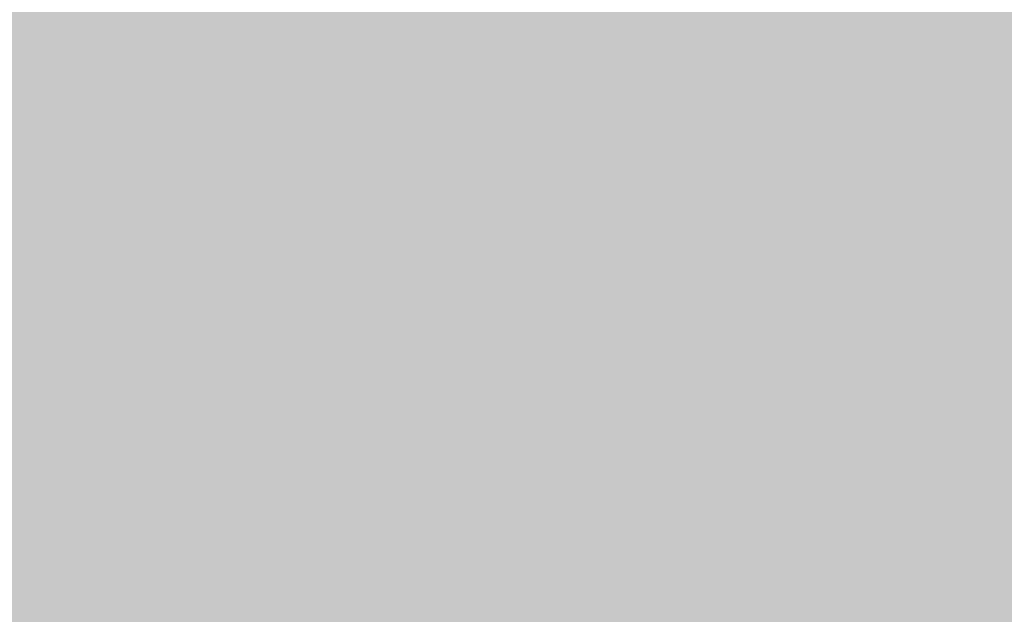
# Model space of a CAD drawing. Units: feet. Extents: x 3168 to 4724, y 827 to 1477.
# Tile 167 of 256: x 3301.945 to 3303.032, y 1098.344 to 1099.001. Entities that reach past the tile are written whole.
import ezdxf

# ---------------------------------------------------------------- set-up
doc = ezdxf.new("R2010")
doc.units = ezdxf.units.FT
doc.layers.add('A-ELEV', color=7, linetype='Continuous', lineweight=35)
doc.layers.add('A-ELEV-PATT', color=8, linetype='Continuous', lineweight=13)

msp = doc.modelspace()

# ---------------------------------------------------------------- hatches: boundary and pattern name
at = {"layer": 'A-ELEV-PATT'}
h = msp.add_hatch(color=256, dxfattribs=at)
h.dxf.hatch_style = 1
edge = h.paths.add_edge_path()
edge.add_ellipse((3552.9058, 979.2201), major_axis=(36.7449, 0), ratio=0.4848485, start_angle=0, end_angle=360)
edge = h.paths.add_edge_path()
edge.add_ellipse((3559.8916, 929.2523), major_axis=(36.7449, 0), ratio=0.4848485, start_angle=0, end_angle=360)
edge = h.paths.add_edge_path()
edge.add_line((3299.3168, 1198.6061), (3479.9167, 1198.6061))
edge.add_line((3479.9167, 1198.6061), (3479.9167, 1209.8686))
edge.add_spline(control_points=[(3479.9167, 1209.8686), (3464.3012, 1209.8686), (3448.6856, 1209.8686), (3410.9491, 1209.8686), (3388.8282, 1209.8686), (3355.6469, 1209.8686), (3344.5864, 1209.8686), (3327.9957, 1209.8686), (3322.4655, 1209.8686), (3314.1702, 1209.8686), (3311.4051, 1209.8686), (3307.2574, 1209.8686), (3305.8748, 1209.8686), (3303.801, 1209.8686), (3303.1097, 1209.8686), (3302.0728, 1209.8686), (3301.7272, 1209.8686), (3301.2087, 1209.8686), (3301.0359, 1209.8686), (3300.7767, 1209.8686), (3300.6903, 1209.8686), (3300.5606, 1209.8686), (3300.5174, 1209.8686), (3300.4526, 1209.8686), (3300.431, 1209.8686), (3300.3986, 1209.8686), (3300.3878, 1209.8686), (3300.3662, 1209.8686), (3300.3457, 1209.8686), (3300.3455, 1209.8686), (3300.3455, 1209.8686), (3300.3433, 1209.8686), (3300.3411, 1209.8686), (3300.3379, 1209.8686), (3300.3368, 1209.8686), (3300.3339, 1209.8686), (3300.3321, 1209.8686), (3300.3255, 1209.8686), (3300.3207, 1209.8686), (3300.3109, 1209.8686), (3300.306, 1209.8686), (3300.2905, 1209.8686), (3300.28, 1209.8686), (3300.2324, 1209.8688), (3300.1953, 1209.869), (3299.9511, 1209.8706), (3299.7448, 1209.8743), (3299.4368, 1209.8833), (3299.3344, 1209.8868), (3299.1811, 1209.8929), (3299.13, 1209.8951), (3298.6522, 1209.9168), (3298.2295, 1209.9457), (3297.6016, 1210.0024), (3297.3934, 1210.0235), (3297.0827, 1210.0583), (3296.9793, 1210.0705), (3296.293, 1210.1549), (3295.7181, 1210.2434), (3294.8687, 1210.3989), (3294.5877, 1210.4545), (3294.1693, 1210.5433), (3294.0304, 1210.5739), (3291.7071, 1211.1012), (3289.6536, 1211.8134), (3285.7763, 1213.564), (3283.9514, 1214.6035), (3280.5122, 1216.9801), (3278.8972, 1218.3176), (3276.3799, 1220.8295), (3275.416, 1221.9177), (3274.0393, 1223.7077), (3273.581, 1224.3495), (3273.1432, 1225.0163)], knot_values=[39.119033, 39.119033, 39.119033, 39.119033, 39.286353, 39.286353, 39.523379, 39.523379, 39.641892, 39.641892, 39.701148, 39.701148, 39.730777, 39.730777, 39.745591, 39.745591, 39.752998, 39.752998, 39.756701, 39.756701, 39.758553, 39.758553, 39.759479, 39.759479, 39.759942, 39.759942, 39.760173, 39.760173, 39.760289, 39.760289, 39.760405, 39.760405, 39.760463, 39.760463, 39.763389, 39.763389, 39.764851, 39.764851, 39.767304, 39.767304, 39.773825, 39.773825, 39.78057, 39.78057, 39.79477, 39.79477, 39.845194, 39.845194, 40.126715, 40.126715, 40.267476, 40.267476, 40.337856, 40.337856, 40.927023, 40.927023, 41.221606, 41.221606, 41.368898, 41.368898, 42.202622, 42.202622, 42.619485, 42.619485, 42.827916, 42.827916, 46.118323, 46.118323, 49.408731, 49.408731, 52.699139, 52.699139, 54.927489, 54.927489, 56.104228, 56.104228, 56.104228, 56.104228], weights=[1, 1, 1, 1, 1, 1, 1, 1, 1, 1, 1, 1, 1, 1, 1, 1, 1, 1, 1, 1, 1, 1, 1, 1, 1, 1, 1, 1, 1, 1, 1, 1, 1, 1, 1, 1, 1, 1, 1, 1, 1, 1, 1, 1, 1, 1, 1, 1, 1, 1, 1, 1, 1, 1, 1, 1, 1, 1, 1, 1, 1, 1, 1, 1, 1, 1, 1, 1, 1, 1, 1, 1, 1, 1], degree=3, periodic=0)
edge.add_line((3273.1432, 1225.0163), (3273.1432, 1099.0163))
edge.add_line((3273.1432, 1099.0163), (3299.3168, 1099.0163))
edge.add_line((3299.3168, 1099.0163), (3299.3168, 1198.6061))
edge = h.paths.add_edge_path()
edge.add_line((3304.7584, 1324.1581), (3479.9167, 1324.1581))
edge.add_line((3479.9167, 1324.1581), (3479.9167, 1335.7146))
edge.add_line((3479.9167, 1335.7146), (3269.1616, 1335.7146))
edge.add_spline(control_points=[(3269.1616, 1335.7146), (3264.0242, 1335.7146), (3258.3641, 1328.9582), (3259.2643, 1323.9003)], knot_values=[0, 0, 0, 0, 15.412191, 15.412191, 15.412191, 15.412191], degree=3, periodic=0)
edge.add_line((3259.2643, 1323.9003), (3265.5168, 1288.7691))
edge.add_line((3265.5168, 1288.7691), (3275.2651, 1261.5456))
edge.add_line((3275.2651, 1261.5456), (3304.7584, 1261.5456))
edge.add_line((3304.7584, 1261.5456), (3304.7584, 1324.1581))
h = msp.add_hatch(color=256, dxfattribs=at)
h.dxf.hatch_style = 1
h.paths.add_polyline_path([(3384.5252, 1099.0163), (3335.0292, 1099.0163), (3299.3168, 1099.0163), (3273.1432, 1099.0163), (3217.5654, 1099.0163), (3168.0693, 827.1163), (3335.0292, 827.1163)])

# ---------------------------------------------------------------- linework, layer by layer
at = {"layer": 'A-ELEV'}
msp.add_open_spline([(3808.5202, 1099.0163), (3808.5202, 1141.4132), (3808.5202, 1183.8102), (3808.5202, 1226.6353), (3808.5202, 1227.0636), (3808.5202, 1227.4918), (3811.4919, 1248.9947), (3814.4635, 1270.4975), (3817.4652, 1292.2176), (3817.4952, 1292.4348), (3817.5253, 1292.652), (3817.5728, 1310.1067), (3817.6203, 1327.5615), (3817.6679, 1345.0163), (3817.6679, 1345.458), (3817.6679, 1345.8996), (3817.6679, 1346.456), (3817.6679, 1346.5708), (3817.6679, 1346.7529), (3817.6679, 1346.8201), (3817.6679, 1346.9349), (3817.6679, 1346.9823), (3817.6679, 1347.0386), (3817.6679, 1347.0474), (3817.6679, 1347.0737), (3817.6679, 1347.0593), (3817.6679, 1347.0615), (3817.6679, 1347.0627), (3817.6679, 1347.066), (3817.6679, 1347.0683), (3817.6679, 1347.075), (3817.6679, 1347.0795), (3817.6678, 1347.0929), (3817.6678, 1347.1019), (3817.6678, 1347.1288), (3817.6677, 1347.1467), (3817.6674, 1347.2004), (3817.6672, 1347.2362), (3817.6661, 1347.3434), (3817.665, 1347.4147), (3817.6608, 1347.6281), (3817.6566, 1347.7697), (3817.64, 1348.1925), (3817.6235, 1348.4716), (3817.5591, 1349.3001), (3817.4961, 1349.8406), (3817.2554, 1351.4242), (3817.0263, 1352.4288), (3816.3069, 1354.8889), (3815.7437, 1356.2687), (3814.464, 1358.8192), (3813.7464, 1359.991), (3812.1958, 1362.1723), (3811.3622, 1363.1821), (3809.5888, 1365.069), (3808.6488, 1365.9461), (3806.6543, 1367.5796), (3805.5997, 1368.3362), (3803.3529, 1369.7223), (3802.1605, 1370.3524), (3799.6008, 1371.4536), (3798.2327, 1371.9255), (3795.2801, 1372.6346), (3793.6931, 1372.8721), (3791.8694, 1372.9265), (3791.7409, 1372.9292), (3791.3534, 1372.9341), (3791.0927, 1372.9329), (3790.3041, 1372.9151), (3789.7695, 1372.8842), (3789.2092, 1372.8302), (3789.1906, 1372.8284), (3789.1349, 1372.8229), (3789.0977, 1372.8191), (3789.0484, 1372.814), (3789.0364, 1372.8127), (3789.0003, 1372.8089), (3788.9761, 1372.8063), (3788.9494, 1372.8034), (3788.9468, 1372.8031), (3788.9426, 1372.8027), (3788.941, 1372.8025), (3788.9386, 1372.8022), (3788.9378, 1372.8021), (3788.9354, 1372.8019), (3788.8675, 1372.7944), (3788.7569, 1372.7822), (3788.7015, 1372.7761), (3788.5355, 1372.7579), (3788.4249, 1372.7457), (3788.0929, 1372.7092), (3787.8715, 1372.6848), (3787.2075, 1372.6118), (3786.7648, 1372.5631), (3785.4368, 1372.417), (3784.5515, 1372.3196), (3781.8954, 1372.0274), (3780.1247, 1371.8327), (3774.8126, 1371.2483), (3771.2713, 1370.8587), (3760.6471, 1369.69), (3753.5643, 1368.9109), (3732.316, 1366.5735), (3718.1504, 1365.0152), (3694.0068, 1362.3593), (3684.0287, 1361.2617), (3674.0506, 1360.1641), (3664.6007, 1360.1641), (3655.1508, 1360.1641), (3626.8011, 1360.1641), (3607.9013, 1360.1641), (3551.2019, 1360.1641), (3513.4023, 1360.1641), (3467.7252, 1360.1641), (3459.8476, 1360.1641), (3436.2149, 1360.1641), (3420.4597, 1360.1641), (3373.1943, 1360.1641), (3341.6839, 1360.1641), (3302.8482, 1360.1641), (3295.5227, 1360.1641), (3286.0383, 1360.1641), (3283.8794, 1360.1641), (3277.4026, 1360.1641), (3273.0848, 1360.1641), (3267.7329, 1360.1641), (3266.6988, 1360.1641), (3263.5965, 1360.1641), (3261.5284, 1360.1641), (3259.2369, 1360.1641), (3259.0137, 1360.1641), (3258.344, 1360.1641), (3257.8975, 1360.1641), (3257.431, 1360.1641), (3257.411, 1360.1641), (3257.3706, 1360.1641), (3257.3755, 1360.1641), (3257.3746, 1360.1641), (3257.3739, 1360.1641), (3257.372, 1360.1641), (3257.3706, 1360.1641), (3257.3667, 1360.1641), (3257.364, 1360.1641), (3257.3561, 1360.1641), (3257.3508, 1360.164), (3257.335, 1360.164), (3257.3244, 1360.164), (3257.2928, 1360.1639), (3257.2717, 1360.1638), (3257.2084, 1360.1634), (3257.1663, 1360.163), (3257.0402, 1360.1614), (3256.9563, 1360.1598), (3256.7055, 1360.1534), (3256.5392, 1360.147), (3256.0436, 1360.1219), (3255.7173, 1360.0971), (3254.7524, 1360.0005), (3254.128, 1359.9065), (3252.1801, 1359.5253), (3250.9416, 1359.144), (3248.6702, 1358.2433), (3247.6357, 1357.7238), (3245.7326, 1356.6035), (3244.8634, 1356.0021), (3243.2531, 1354.7429), (3242.512, 1354.0847), (3240.7511, 1352.3448), (3239.801, 1351.2296), (3238.0878, 1348.8724), (3237.3247, 1347.6304), (3235.9825, 1344.9716), (3235.4022, 1343.5549), (3234.5911, 1340.8155), (3234.3109, 1339.5435), (3233.9765, 1336.8026), (3233.9221, 1335.3309), (3234.1489, 1332.5913), (3234.3495, 1331.3672), (3234.7199, 1329.9994), (3234.7524, 1329.8834), (3234.8536, 1329.5348), (3234.9259, 1329.3017), (3235.0248, 1329.0026), (3235.0469, 1328.9369), (3235.0776, 1328.8472), (3235.0859, 1328.8232), (3235.1109, 1328.7511), (3235.1278, 1328.703), (3235.148, 1328.6462), (3235.1511, 1328.6376), (3235.1561, 1328.6235), (3235.1581, 1328.618), (3235.1602, 1328.612), (3235.1656, 1328.5969), (3235.1801, 1328.5565), (3235.1903, 1328.5281), (3235.2208, 1328.4429), (3235.2411, 1328.3862), (3235.3021, 1328.2159), (3235.3427, 1328.1023), (3235.4647, 1327.7617), (3235.546, 1327.5346), (3235.79, 1326.8534), (3235.9526, 1326.3992), (3236.4405, 1325.0367), (3236.7657, 1324.1284), (3237.7415, 1321.4034), (3238.392, 1319.5868), (3240.3435, 1314.1369), (3241.6445, 1310.5036), (3245.5476, 1299.6037), (3248.1496, 1292.3371), (3255.9557, 1270.5374), (3261.1598, 1256.0042), (3267.3876, 1238.612), (3268.4114, 1235.7529), (3269.5104, 1232.6839), (3269.5856, 1232.4739), (3269.7066, 1232.1359), (3269.7524, 1232.0079), (3269.8273, 1231.7987), (3269.8564, 1231.7176), (3269.9063, 1231.5781), (3269.9272, 1231.5198), (3269.9725, 1231.3934), (3269.9968, 1231.3254), (3270.0265, 1231.2425), (3270.0318, 1231.2277), (3270.0403, 1231.204), (3270.0392, 1231.207), (3270.0394, 1231.2066), (3270.0394, 1231.2064), (3270.0396, 1231.2058), (3270.0398, 1231.2055), (3270.0402, 1231.2043), (3270.0404, 1231.2036), (3270.0413, 1231.2013), (3270.0418, 1231.1998), (3270.0434, 1231.1953), (3270.0445, 1231.1922), (3270.0478, 1231.1832), (3270.0499, 1231.1771), (3270.0564, 1231.159), (3270.0608, 1231.147), (3270.0739, 1231.1108), (3270.0826, 1231.0867), (3270.1089, 1231.0144), (3270.1266, 1230.9663), (3270.1799, 1230.8225), (3270.2159, 1230.7269), (3270.3253, 1230.4415), (3270.4, 1230.2528), (3270.6292, 1229.6914), (3270.7889, 1229.3235), (3271.2865, 1228.2383), (3271.6431, 1227.5398), (3272.7759, 1225.5153), (3273.6142, 1224.2605), (3275.416, 1221.9177), (3276.3799, 1220.8295), (3278.8972, 1218.3176), (3280.5122, 1216.9801), (3283.9514, 1214.6035), (3285.7763, 1213.564), (3289.6536, 1211.8134), (3291.7071, 1211.1012), (3294.0304, 1210.5739), (3294.1693, 1210.5433), (3294.5877, 1210.4545), (3294.8687, 1210.3989), (3295.7181, 1210.2434), (3296.293, 1210.1549), (3296.9793, 1210.0705), (3297.0827, 1210.0583), (3297.3934, 1210.0235), (3297.6016, 1210.0024), (3298.2295, 1209.9457), (3298.6522, 1209.9168), (3299.13, 1209.8951), (3299.1811, 1209.8929), (3299.3344, 1209.8868), (3299.4368, 1209.8833), (3299.7448, 1209.8743), (3299.9511, 1209.8706), (3300.1953, 1209.869), (3300.2324, 1209.8688), (3300.28, 1209.8686), (3300.2905, 1209.8686), (3300.306, 1209.8686), (3300.3109, 1209.8686), (3300.3207, 1209.8686), (3300.3255, 1209.8686), (3300.3321, 1209.8686), (3300.3339, 1209.8686), (3300.3368, 1209.8686), (3300.3379, 1209.8686), (3300.3411, 1209.8686), (3300.3433, 1209.8686), (3300.3455, 1209.8686), (3300.3455, 1209.8686), (3300.3457, 1209.8686), (3300.3662, 1209.8686), (3300.3878, 1209.8686), (3300.3986, 1209.8686), (3300.431, 1209.8686), (3300.4526, 1209.8686), (3300.5174, 1209.8686), (3300.5606, 1209.8686), (3300.6903, 1209.8686), (3300.7767, 1209.8686), (3301.0359, 1209.8686), (3301.2087, 1209.8686), (3301.7272, 1209.8686), (3302.0728, 1209.8686), (3303.1097, 1209.8686), (3303.801, 1209.8686), (3305.8748, 1209.8686), (3307.2574, 1209.8686), (3311.4051, 1209.8686), (3314.1702, 1209.8686), (3322.4655, 1209.8686), (3327.9957, 1209.8686), (3344.5864, 1209.8686), (3355.6469, 1209.8686), (3388.8282, 1209.8686), (3410.9491, 1209.8686), (3477.3119, 1209.8686), (3521.5537, 1209.8686), (3566.8362, 1209.8686), (3567.8769, 1209.8686), (3570.999, 1209.8686), (3573.0804, 1209.8686), (3575.7814, 1209.8686), (3576.4009, 1209.8686), (3577.2958, 1209.8686), (3577.5712, 1209.8686), (3578.3971, 1209.8686), (3578.9478, 1209.8686), (3579.7565, 1209.8686), (3580.0145, 1209.8686), (3580.3427, 1209.8686), (3580.3269, 1209.8686), (3580.3272, 1209.8686), (3580.3273, 1209.8686), (3580.3278, 1209.8686), (3580.3281, 1209.8686), (3580.329, 1209.8686), (3580.3296, 1209.8686), (3580.3314, 1209.8686), (3580.3327, 1209.8686), (3580.3363, 1209.8686), (3580.3388, 1209.8686), (3580.3461, 1209.8686), (3580.351, 1209.8686), (3580.3657, 1209.8685), (3580.3754, 1209.8685), (3580.4048, 1209.8684), (3580.4244, 1209.8684), (3580.4832, 1209.8681), (3580.5224, 1209.8678), (3580.6404, 1209.8666), (3580.7192, 1209.8655), (3580.9563, 1209.8608), (3581.1152, 1209.8561), (3581.5942, 1209.8372), (3581.9164, 1209.8183), (3582.8899, 1209.7424), (3583.548, 1209.6662), (3585.5318, 1209.3606), (3586.8672, 1209.0539), (3589.4715, 1208.2525), (3590.7402, 1207.7579), (3591.9955, 1207.1588), (3592.0578, 1207.1287), (3592.2442, 1207.038), (3592.3677, 1206.9766), (3592.7353, 1206.7904), (3592.9768, 1206.6631), (3593.2445, 1206.5164), (3593.2747, 1206.4998), (3593.3651, 1206.4498), (3593.4251, 1206.4163), (3593.6043, 1206.3153), (3593.7227, 1206.2472), (3593.8572, 1206.1684), (3593.8744, 1206.1583), (3593.9257, 1206.128), (3593.9599, 1206.1078), (3594.0621, 1206.0469), (3594.1298, 1206.0061), (3594.2084, 1205.9582), (3594.2197, 1205.9513), (3594.2534, 1205.9307), (3594.2758, 1205.9169), (3594.343, 1205.8755), (3594.3876, 1205.8479), (3594.4336, 1205.819), (3594.4353, 1205.818), (3594.4402, 1205.8149), (3594.4435, 1205.8129), (3594.4471, 1205.8106), (3594.4475, 1205.8103), (3594.4487, 1205.8096), (3594.4495, 1205.8091), (3594.4504, 1205.8086), (3594.4505, 1205.8085), (3594.4506, 1205.8084), (3594.4674, 1205.7979), (3594.4933, 1205.7817), (3594.5062, 1205.7736), (3594.545, 1205.7492), (3594.5709, 1205.733), (3594.6485, 1205.6844), (3594.7002, 1205.652), (3594.8554, 1205.5547), (3594.9589, 1205.4898), (3595.2694, 1205.2953), (3595.4763, 1205.1656), (3596.0972, 1204.7765), (3596.5111, 1204.5171), (3597.7528, 1203.7388), (3598.5807, 1203.22), (3601.0642, 1201.6636), (3602.7198, 1200.6259), (3607.6868, 1197.513), (3610.9981, 1195.4377), (3620.932, 1189.2119), (3627.5546, 1185.0614), (3647.4225, 1172.6097), (3660.6678, 1164.3086), (3700.4035, 1139.4053), (3726.894, 1122.8031), (3757.2057, 1103.8061), (3761.027, 1101.4112), (3764.8482, 1099.0163), (3745.3283, 1099.0163), (3725.8083, 1099.0163), (3706.2884, 1099.0163), (3706.2884, 1108.4532), (3706.2884, 1117.8902), (3706.2884, 1127.3271), (3710.7508, 1127.3271), (3715.2131, 1127.3271), (3719.6755, 1127.3271)], degree=3, knots=[0, 0, 0, 0, 0.982037, 0.982037, 0.991957, 0.991957, 0.991957, 1.966522, 1.966522, 1.976367, 1.976367, 1.976367, 2.976367, 2.976367, 2.976367, 3.00169, 3.00169, 3.008272, 3.008272, 3.012129, 3.012129, 3.014851, 3.014851, 3.015353, 3.015353, 3.016359, 3.016359, 3.017365, 3.017365, 3.019376, 3.019376, 3.023398, 3.023398, 3.031442, 3.031442, 3.047531, 3.047531, 3.079708, 3.079708, 3.144063, 3.144063, 3.272772, 3.272772, 3.53019, 3.53019, 4.045026, 4.045026, 5.074698, 5.074698, 6.700878, 6.700878, 8.327058, 8.327058, 9.953238, 9.953238, 11.579418, 11.579418, 13.205598, 13.205598, 14.831778, 14.831778, 16.457958, 16.457958, 18.084138, 18.084138, 18.206872, 18.206872, 18.45234, 18.45234, 18.943275, 18.943275, 18.960093, 18.960093, 18.993729, 18.993729, 19.00461, 19.00461, 19.026374, 19.026374, 19.028737, 19.028737, 19.03018, 19.03018, 19.030897, 19.030897, 19.032332, 19.032332, 19.033766, 19.033766, 19.036636, 19.036636, 19.042374, 19.042374, 19.053851, 19.053851, 19.076805, 19.076805, 19.122714, 19.122714, 19.21453, 19.21453, 19.398163, 19.398163, 19.765429, 19.765429, 20.024128, 20.024128, 20.024128, 20.092031, 20.092031, 20.227836, 20.227836, 20.499446, 20.499446, 20.556051, 20.556051, 20.66926, 20.66926, 20.895678, 20.895678, 20.948316, 20.948316, 20.963829, 20.963829, 20.994855, 20.994855, 21.002285, 21.002285, 21.017146, 21.017146, 21.01875, 21.01875, 21.021959, 21.021959, 21.022102, 21.022102, 21.022249, 21.022249, 21.022708, 21.022708, 21.023627, 21.023627, 21.025464, 21.025464, 21.029138, 21.029138, 21.036486, 21.036486, 21.051183, 21.051183, 21.080575, 21.080575, 21.139361, 21.139361, 21.256932, 21.256932, 21.492073, 21.492073, 21.962356, 21.962356, 23.01002, 23.01002, 24.057684, 24.057684, 25.105348, 25.105348, 26.153011, 26.153011, 27.776787, 27.776787, 29.400562, 29.400562, 31.024337, 31.024337, 32.278801, 32.278801, 33.533265, 33.533265, 34.467568, 34.467568, 34.553971, 34.553971, 34.726776, 34.726776, 34.775309, 34.775309, 34.793079, 34.793079, 34.82862, 34.82862, 34.834979, 34.834979, 34.839039, 34.839039, 34.839411, 34.839411, 34.840285, 34.840285, 34.842034, 34.842034, 34.845531, 34.845531, 34.852525, 34.852525, 34.866512, 34.866512, 34.894488, 34.894488, 34.950439, 34.950439, 35.062342, 35.062342, 35.286147, 35.286147, 35.733758, 35.733758, 35.821815, 35.821815, 35.828283, 35.828283, 35.832225, 35.832225, 35.834724, 35.834724, 35.836521, 35.836521, 35.838617, 35.838617, 35.839073, 35.839073, 35.839345, 35.839345, 35.839617, 35.839617, 35.840161, 35.840161, 35.841249, 35.841249, 35.843425, 35.843425, 35.847778, 35.847778, 35.856482, 35.856482, 35.873891, 35.873891, 35.908709, 35.908709, 35.978345, 35.978345, 36.117617, 36.117617, 36.396161, 36.396161, 36.953248, 36.953248, 38.067423, 38.067423, 40.295772, 40.295772, 42.524122, 42.524122, 45.81453, 45.81453, 49.104937, 49.104937, 52.395345, 52.395345, 52.603776, 52.603776, 53.020639, 53.020639, 53.854363, 53.854363, 54.001655, 54.001655, 54.296238, 54.296238, 54.885405, 54.885405, 54.955785, 54.955785, 55.096546, 55.096546, 55.378067, 55.378067, 55.42849, 55.42849, 55.442691, 55.442691, 55.449436, 55.449436, 55.455957, 55.455957, 55.458409, 55.458409, 55.459872, 55.459872, 55.462798, 55.462798, 55.462856, 55.462856, 55.462972, 55.462972, 55.463088, 55.463088, 55.463319, 55.463319, 55.463782, 55.463782, 55.464708, 55.464708, 55.46656, 55.46656, 55.470263, 55.470263, 55.47767, 55.47767, 55.492484, 55.492484, 55.522112, 55.522112, 55.581369, 55.581369, 55.699882, 55.699882, 55.936907, 55.936907, 56.410959, 56.410959, 56.42211, 56.42211, 56.444413, 56.444413, 56.451051, 56.451051, 56.454001, 56.454001, 56.459901, 56.459901, 56.462666, 56.462666, 56.463418, 56.463418, 56.464171, 56.464171, 56.465675, 56.465675, 56.468684, 56.468684, 56.474702, 56.474702, 56.486738, 56.486738, 56.51081, 56.51081, 56.558955, 56.558955, 56.655243, 56.655243, 56.847821, 56.847821, 57.232975, 57.232975, 58.003284, 58.003284, 59.543901, 59.543901, 62.625137, 62.625137, 68.787607, 68.787607, 74.950078, 74.950078, 75.27336, 75.27336, 75.919923, 75.919923, 77.213051, 77.213051, 77.377769, 77.377769, 77.707206, 77.707206, 78.366079, 78.366079, 78.462532, 78.462532, 78.655436, 78.655436, 79.041245, 79.041245, 79.105735, 79.105735, 79.234714, 79.234714, 79.492672, 79.492672, 79.502197, 79.502197, 79.521249, 79.521249, 79.523534, 79.523534, 79.528103, 79.528103, 79.528682, 79.528682, 79.528885, 79.528885, 79.529089, 79.529089, 79.529495, 79.529495, 79.530308, 79.530308, 79.531935, 79.531935, 79.535187, 79.535187, 79.541693, 79.541693, 79.554704, 79.554704, 79.580725, 79.580725, 79.632769, 79.632769, 79.736856, 79.736856, 79.94503, 79.94503, 80.361377, 80.361377, 80.421435, 80.421435, 80.421435, 81.421435, 81.421435, 81.421435, 82.421435, 82.421435, 82.421435, 83.421435, 83.421435, 83.421435, 83.421435], dxfattribs=at)

doc.saveas('drawing.dxf')
